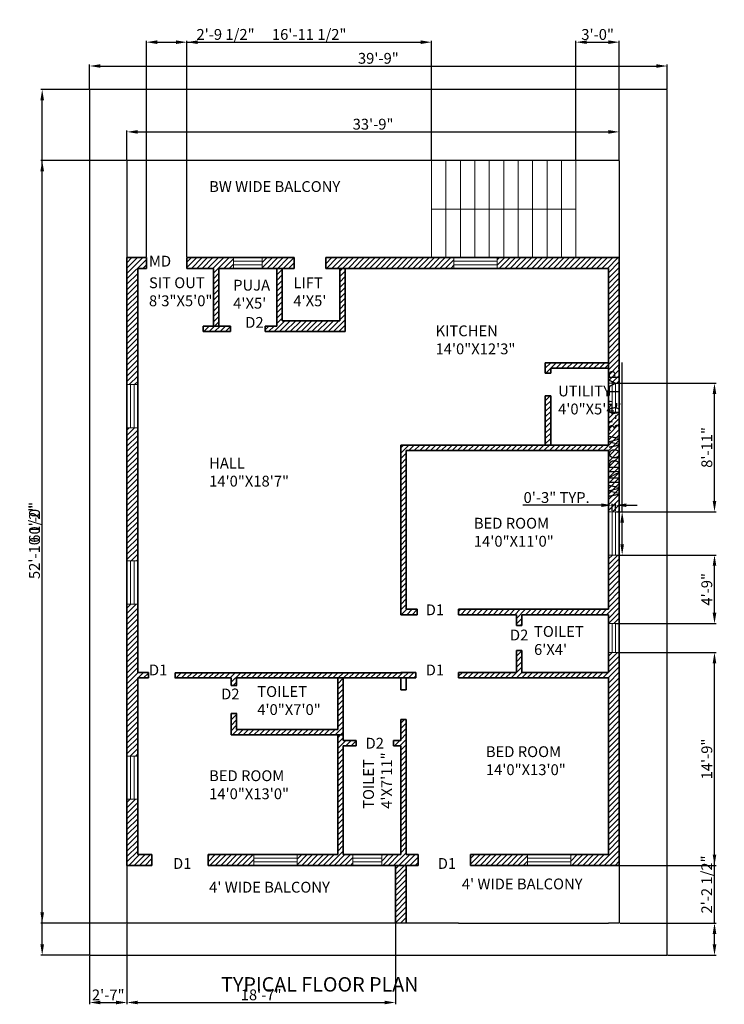
# Model space of a CAD drawing. Units: inches. Extents: x 9573 to 10767, y 4927 to 5746.
# Tile 1 of 2: x 9573 to 10158, y 4927 to 5746. Entities that reach past the tile are written whole.
import ezdxf

# ---------------------------------------------------------------- set-up
doc = ezdxf.new("R2010")
doc.units = ezdxf.units.IN
for name, color, linetype, lineweight in [('A-ANNO-DIMS', 2, 'Continuous', 18), ('A-ANNO-TEXT', 7, 'Continuous', 25), ('A-AREA-IDEN', 7, 'Continuous', 18), ('A-DOOR-IDEN', 3, 'Continuous', 18), ('A-FLOR-BALC', 7, 'Continuous', 25), ('A-FLOR-STRS', 7, 'Continuous', 18), ('A-GLAZ', 4, 'Continuous', 18), ('A-WALL', 7, 'Continuous', 35), ('A-WALL-PATT', 252, 'Continuous', 13), ('C-PROP', 8, 'Continuous', 25)]:
    doc.layers.add(name, color=color, linetype=linetype, lineweight=lineweight)
doc.styles.get("Standard").update_dxf_attribs({"font": 'arial.ttf'})
doc.dimstyles.new('ISO-25', dxfattribs={"dimtxt": 9, "dimasz": 9, "dimexe": 1.25, "dimexo": 0.625, "dimtad": 1, "dimdec": 1, "dimrnd": 9, "dimlunit": 3, "dimtxsty": 'Standard', "dimcen": 2.5, "dimadec": 0, "dimazin": 0, "dimtfac": 1, "dimtdec": 1, "dimtmove": 0, "dimatfit": 3, "dimfxl": 1, "dimarcsym": 0})

# ---------------------------------------------------------------- blocks, each defined once
blk = doc.blocks.new('*D1')
at = {"layer": 'A-ANNO-DIMS', "color": 0, "lineweight": -2, "transparency": 16777216}
for p, q in [((9661.65, 5629.81), (9661.65, 5654.25)), ((9670.65, 5653), (10061.84, 5653)), ((10070.84, 5629.81), (10070.84, 5654.25))]:
    blk.add_line(p, q, dxfattribs=at)
at = {"layer": 'A-ANNO-DIMS', "color": 0, "transparency": 16777216}
for points in [[(9670.65, 5654.5), (9670.65, 5651.5), (9661.65, 5653)], [(10061.84, 5654.5), (10061.84, 5651.5), (10070.84, 5653)]]:
    blk.add_solid(points, dxfattribs=at)
at = {"layer": 'Defpoints', "color": 0, "transparency": 16777216}
for p in [(10070.84, 5653), (9661.65, 5629.18), (10070.84, 5629.18)]:
    blk.add_point(p, dxfattribs=at)
at = {"layer": 'A-ANNO-DIMS', "color": 0, "transparency": 16777216, "insert": (9866.24, 5658.23), "char_height": 9, "attachment_point": 5}
blk.add_mtext('33\'-9"', dxfattribs=at)
blk = doc.blocks.new('*D2')
at = {"layer": 'A-ANNO-DIMS', "color": 0, "lineweight": -2, "transparency": 16777216}
for p, q in [((9630.63, 5688.89), (9630.63, 5709.04)), ((9639.63, 5707.79), (10101.63, 5707.79)), ((10110.63, 5688.89), (10110.63, 5709.04))]:
    blk.add_line(p, q, dxfattribs=at)
at = {"layer": 'A-ANNO-DIMS', "color": 0, "transparency": 16777216}
for points in [[(9639.63, 5709.29), (9639.63, 5706.29), (9630.63, 5707.79)], [(10101.63, 5709.29), (10101.63, 5706.29), (10110.63, 5707.79)]]:
    blk.add_solid(points, dxfattribs=at)
at = {"layer": 'Defpoints', "color": 0, "transparency": 16777216}
for p in [(10110.63, 5707.79), (9630.63, 5688.26), (10110.63, 5688.26)]:
    blk.add_point(p, dxfattribs=at)
at = {"layer": 'A-ANNO-DIMS', "color": 0, "transparency": 16777216, "insert": (9870.63, 5713.01), "char_height": 9, "attachment_point": 5}
blk.add_mtext('39\'-9"', dxfattribs=at)
blk = doc.blocks.new('GLAZ-36IN')
for p, q in [((0, 3), (36, 3)), ((0, 0), (36, 0))]:
    blk.add_line(p, q)
blk = doc.blocks.new('GLAZ-24IN')
for p, q in [((0, 3), (24, 3)), ((0, 0), (24, 0))]:
    blk.add_line(p, q)
blk = doc.blocks.new('STAIR-TWIN-FLIGHT')
for p, q in [((0, 80.77), (0, 0)), ((12, 80.77), (12, 0)), ((24, 80.77), (24, 0)), ((36, 80.77), (36, 0)), ((48, 80.77), (48, 0)), ((60, 80.77), (60, 0)), ((72, 80.77), (72, 0)), ((84, 80.77), (84, 0)), ((96, 80.77), (96, 0)), ((108, 80.77), (108, 0)), ((120, 80.77), (120, 0)), ((0, 40.39), (120, 40.39))]:
    blk.add_line(p, q)
blk = doc.blocks.new('*D8')
at = {"layer": 'A-ANNO-DIMS', "color": 0, "lineweight": -2, "transparency": 16777216}
for p, q in [((10073.24, 5337.09), (10073.24, 5461.23)), ((10068.46, 5337.09), (10074.49, 5337.09)), ((10073.24, 5310.09), (10073.24, 5328.09)), ((10068.46, 5301.09), (10074.49, 5301.09))]:
    blk.add_line(p, q, dxfattribs=at)
at = {"layer": 'A-ANNO-DIMS', "color": 0, "transparency": 16777216}
for points in [[(10071.74, 5328.09), (10074.74, 5328.09), (10073.24, 5337.09)], [(10071.74, 5310.09), (10074.74, 5310.09), (10073.24, 5301.09)]]:
    blk.add_solid(points, dxfattribs=at)
at = {"layer": 'Defpoints', "color": 0, "transparency": 16777216}
for p in [(10067.84, 5337.09), (10073.24, 5337.09), (10067.84, 5301.09)]:
    blk.add_point(p, dxfattribs=at)
at = {"layer": 'A-ANNO-DIMS', "color": 0, "transparency": 16777216, "insert": (10067.95, 5403.66), "char_height": 9, "attachment_point": 5, "rotation": 90}
blk.add_mtext('WINDOW 3\'-0" TYP.', dxfattribs=at)
blk = doc.blocks.new('*D9')
at = {"layer": 'A-ANNO-DIMS', "color": 0, "lineweight": -2, "transparency": 16777216}
for p, q in [((10055.84, 5342.49), (9990.73, 5342.49)), ((10064.84, 5337.72), (10064.84, 5343.74)), ((10067.84, 5342.49), (10064.84, 5342.49)), ((10067.84, 5337.72), (10067.84, 5343.74)), ((10076.84, 5342.49), (10085.84, 5342.49))]:
    blk.add_line(p, q, dxfattribs=at)
at = {"layer": 'A-ANNO-DIMS', "color": 0, "transparency": 16777216}
for points in [[(10055.84, 5343.99), (10055.84, 5340.99), (10064.84, 5342.49)], [(10076.84, 5343.99), (10076.84, 5340.99), (10067.84, 5342.49)]]:
    blk.add_solid(points, dxfattribs=at)
at = {"layer": 'Defpoints', "color": 0, "transparency": 16777216}
for p in [(10064.84, 5342.49), (10064.84, 5337.09), (10067.84, 5337.09)]:
    blk.add_point(p, dxfattribs=at)
at = {"layer": 'A-ANNO-DIMS', "color": 0, "transparency": 16777216, "insert": (10018.78, 5347.72), "char_height": 9, "attachment_point": 5}
blk.add_mtext('0\'-3" TYP.', dxfattribs=at)
blk = doc.blocks.new('*D14')
at = {"layer": 'A-ANNO-DIMS', "color": 0, "lineweight": -2, "transparency": 16777216}
for p, q in [((9661.02, 5629.18), (9590.03, 5629.18)), ((9591.28, 5003.91), (9591.28, 5620.18)), ((9661.02, 4994.91), (9590.03, 4994.91))]:
    blk.add_line(p, q, dxfattribs=at)
at = {"layer": 'A-ANNO-DIMS', "color": 0, "transparency": 16777216}
for points in [[(9589.78, 5620.18), (9592.78, 5620.18), (9591.28, 5629.18)], [(9589.78, 5003.91), (9592.78, 5003.91), (9591.28, 4994.91)]]:
    blk.add_solid(points, dxfattribs=at)
at = {"layer": 'Defpoints', "color": 0, "transparency": 16777216}
for p in [(9591.28, 5629.18), (9661.65, 5629.18), (9661.65, 4994.91)]:
    blk.add_point(p, dxfattribs=at)
at = {"layer": 'A-ANNO-DIMS', "color": 0, "transparency": 16777216, "insert": (9586, 5312.05), "char_height": 9, "attachment_point": 5, "rotation": 90}
blk.add_mtext('52\'-10 1/2"', dxfattribs=at)
blk = doc.blocks.new('*D15')
at = {"layer": 'A-ANNO-DIMS', "color": 0, "lineweight": -2, "transparency": 16777216}
for p, q in [((9630, 5688.26), (9590.03, 5688.26)), ((9591.28, 4977.26), (9591.28, 5679.26)), ((9630, 4968.26), (9590.03, 4968.26))]:
    blk.add_line(p, q, dxfattribs=at)
at = {"layer": 'A-ANNO-DIMS', "color": 0, "transparency": 16777216}
for points in [[(9589.78, 5679.26), (9592.78, 5679.26), (9591.28, 5688.26)], [(9589.78, 4977.26), (9592.78, 4977.26), (9591.28, 4968.26)]]:
    blk.add_solid(points, dxfattribs=at)
at = {"layer": 'Defpoints', "color": 0, "transparency": 16777216}
for p in [(9591.28, 5688.26), (9630.63, 5688.26), (9630.63, 4968.26)]:
    blk.add_point(p, dxfattribs=at)
at = {"layer": 'A-ANNO-DIMS', "color": 0, "transparency": 16777216, "insert": (9586.06, 5328.26), "char_height": 9, "attachment_point": 5, "rotation": 90}
blk.add_mtext('60\'-0"', dxfattribs=at)
blk = doc.blocks.new('*D16')
at = {"layer": 'A-ANNO-DIMS', "color": 0, "lineweight": -2, "transparency": 16777216}
for p, q in [((9661.65, 4994.28), (9661.65, 4927.66)), ((9630.63, 4967.64), (9630.63, 4927.66)), ((9639.63, 4928.91), (9652.65, 4928.91))]:
    blk.add_line(p, q, dxfattribs=at)
at = {"layer": 'A-ANNO-DIMS', "color": 0, "transparency": 16777216}
for points in [[(9639.63, 4930.41), (9639.63, 4927.41), (9630.63, 4928.91)], [(9652.65, 4930.41), (9652.65, 4927.41), (9661.65, 4928.91)]]:
    blk.add_solid(points, dxfattribs=at)
at = {"layer": 'Defpoints', "color": 0, "transparency": 16777216}
for p in [(9661.65, 4994.91), (9630.63, 4968.26), (9661.65, 4928.91)]:
    blk.add_point(p, dxfattribs=at)
at = {"layer": 'A-ANNO-DIMS', "color": 0, "transparency": 16777216, "insert": (9646.14, 4934.06), "char_height": 9, "attachment_point": 5}
blk.add_mtext('2\'-7"', dxfattribs=at)
blk = doc.blocks.new('*D17')
at = {"layer": 'A-ANNO-DIMS', "color": 0, "lineweight": -2, "transparency": 16777216}
for p, q in [((10149.98, 4994.91), (10149.98, 5050.21)), ((10071.46, 4994.91), (10151.23, 4994.91)), ((10149.98, 4977.26), (10149.98, 4985.91)), ((10111.25, 4968.26), (10151.23, 4968.26))]:
    blk.add_line(p, q, dxfattribs=at)
at = {"layer": 'A-ANNO-DIMS', "color": 0, "transparency": 16777216}
for points in [[(10148.48, 4985.91), (10151.48, 4985.91), (10149.98, 4994.91)], [(10148.48, 4977.26), (10151.48, 4977.26), (10149.98, 4968.26)]]:
    blk.add_solid(points, dxfattribs=at)
at = {"layer": 'Defpoints', "color": 0, "transparency": 16777216}
for p in [(10070.84, 4994.91), (10149.98, 4994.91), (10110.63, 4968.26)]:
    blk.add_point(p, dxfattribs=at)
at = {"layer": 'A-ANNO-DIMS', "color": 0, "transparency": 16777216, "insert": (10144.7, 5027.06), "char_height": 9, "attachment_point": 5, "rotation": 90}
blk.add_mtext('2\'-2 1/2"', dxfattribs=at)
blk = doc.blocks.new('*D22')
at = {"layer": 'A-ANNO-DIMS', "color": 0, "lineweight": -2, "transparency": 16777216}
for p, q in [((10034.84, 5629.81), (10034.84, 5728.86)), ((10043.84, 5727.61), (10061.84, 5727.61)), ((10070.84, 5629.81), (10070.84, 5728.86))]:
    blk.add_line(p, q, dxfattribs=at)
at = {"layer": 'A-ANNO-DIMS', "color": 0, "transparency": 16777216}
for points in [[(10043.84, 5729.11), (10043.84, 5726.11), (10034.84, 5727.61)], [(10061.84, 5729.11), (10061.84, 5726.11), (10070.84, 5727.61)]]:
    blk.add_solid(points, dxfattribs=at)
at = {"layer": 'Defpoints', "color": 0, "transparency": 16777216}
for p in [(10070.84, 5727.61), (10034.84, 5629.18), (10070.84, 5629.18)]:
    blk.add_point(p, dxfattribs=at)
at = {"layer": 'A-ANNO-DIMS', "color": 0, "transparency": 16777216, "insert": (10052.84, 5732.83), "char_height": 9, "attachment_point": 5}
blk.add_mtext('3\'-0"', dxfattribs=at)
blk = doc.blocks.new('*D24')
at = {"layer": 'A-ANNO-DIMS', "color": 0, "lineweight": -2, "transparency": 16777216}
for p, q in [((9677.83, 5549.03), (9677.83, 5728.86)), ((9686.83, 5727.61), (9702.46, 5727.61)), ((9711.46, 5549.03), (9711.46, 5728.86)), ((9711.46, 5727.61), (9766.76, 5727.61))]:
    blk.add_line(p, q, dxfattribs=at)
at = {"layer": 'A-ANNO-DIMS', "color": 0, "transparency": 16777216}
for points in [[(9686.83, 5729.11), (9686.83, 5726.11), (9677.83, 5727.61)], [(9702.46, 5729.11), (9702.46, 5726.11), (9711.46, 5727.61)]]:
    blk.add_solid(points, dxfattribs=at)
at = {"layer": 'Defpoints', "color": 0, "transparency": 16777216}
for p in [(9711.46, 5727.61), (9677.83, 5548.41), (9711.46, 5548.41)]:
    blk.add_point(p, dxfattribs=at)
at = {"layer": 'A-ANNO-DIMS', "color": 0, "transparency": 16777216, "insert": (9743.61, 5732.89), "char_height": 9, "attachment_point": 5}
blk.add_mtext('2\'-9 1/2"', dxfattribs=at)
blk = doc.blocks.new('*D25')
at = {"layer": 'A-ANNO-DIMS', "color": 0, "lineweight": -2, "transparency": 16777216}
for p, q in [((9711.46, 5549.03), (9711.46, 5728.86)), ((9720.46, 5727.61), (9905.84, 5727.61)), ((9914.84, 5629.81), (9914.84, 5728.86))]:
    blk.add_line(p, q, dxfattribs=at)
at = {"layer": 'A-ANNO-DIMS', "color": 0, "transparency": 16777216}
for points in [[(9720.46, 5729.11), (9720.46, 5726.11), (9711.46, 5727.61)], [(9905.84, 5729.11), (9905.84, 5726.11), (9914.84, 5727.61)]]:
    blk.add_solid(points, dxfattribs=at)
at = {"layer": 'Defpoints', "color": 0, "transparency": 16777216}
for p in [(9914.84, 5727.61), (9914.84, 5629.18), (9711.46, 5548.41)]:
    blk.add_point(p, dxfattribs=at)
at = {"layer": 'A-ANNO-DIMS', "color": 0, "transparency": 16777216, "insert": (9813.15, 5732.89), "char_height": 9, "attachment_point": 5}
blk.add_mtext('16\'-11 1/2"', dxfattribs=at)
blk = doc.blocks.new('*D28')
at = {"layer": 'A-ANNO-DIMS', "color": 0, "lineweight": -2, "transparency": 16777216}
for p, q in [((10068.46, 5220), (10151.23, 5220)), ((10149.98, 5051.91), (10149.98, 5211)), ((10071.46, 5042.91), (10151.23, 5042.91))]:
    blk.add_line(p, q, dxfattribs=at)
at = {"layer": 'A-ANNO-DIMS', "color": 0, "transparency": 16777216}
for points in [[(10148.48, 5211), (10151.48, 5211), (10149.98, 5220)], [(10148.48, 5051.91), (10151.48, 5051.91), (10149.98, 5042.91)]]:
    blk.add_solid(points, dxfattribs=at)
at = {"layer": 'Defpoints', "color": 0, "transparency": 16777216}
for p in [(10067.84, 5220), (10149.98, 5220), (10070.84, 5042.91)]:
    blk.add_point(p, dxfattribs=at)
at = {"layer": 'A-ANNO-DIMS', "color": 0, "transparency": 16777216, "insert": (10144.76, 5131.45), "char_height": 9, "attachment_point": 5, "rotation": 90}
blk.add_mtext('14\'-9"', dxfattribs=at)
blk = doc.blocks.new('*D29')
at = {"layer": 'A-ANNO-DIMS', "color": 0, "lineweight": -2, "transparency": 16777216}
for p, q in [((10068.46, 5301.09), (10151.23, 5301.09)), ((10149.98, 5253), (10149.98, 5292.09)), ((10068.46, 5244), (10151.23, 5244))]:
    blk.add_line(p, q, dxfattribs=at)
at = {"layer": 'A-ANNO-DIMS', "color": 0, "transparency": 16777216}
for points in [[(10148.48, 5292.09), (10151.48, 5292.09), (10149.98, 5301.09)], [(10148.48, 5253), (10151.48, 5253), (10149.98, 5244)]]:
    blk.add_solid(points, dxfattribs=at)
at = {"layer": 'Defpoints', "color": 0, "transparency": 16777216}
for p in [(10067.84, 5301.09), (10149.98, 5301.09), (10067.84, 5244)]:
    blk.add_point(p, dxfattribs=at)
at = {"layer": 'A-ANNO-DIMS', "color": 0, "transparency": 16777216, "insert": (10144.76, 5272.55), "char_height": 9, "attachment_point": 5, "rotation": 90}
blk.add_mtext('4\'-9"', dxfattribs=at)
blk = doc.blocks.new('*D30')
at = {"layer": 'A-ANNO-DIMS', "color": 0, "lineweight": -2, "transparency": 16777216}
for p, q in [((10068.46, 5444), (10151.23, 5444)), ((10149.98, 5346.09), (10149.98, 5435)), ((10068.46, 5337.09), (10151.23, 5337.09))]:
    blk.add_line(p, q, dxfattribs=at)
at = {"layer": 'A-ANNO-DIMS', "color": 0, "transparency": 16777216}
for points in [[(10148.48, 5435), (10151.48, 5435), (10149.98, 5444)], [(10148.48, 5346.09), (10151.48, 5346.09), (10149.98, 5337.09)]]:
    blk.add_solid(points, dxfattribs=at)
at = {"layer": 'Defpoints', "color": 0, "transparency": 16777216}
for p in [(10067.84, 5444), (10149.98, 5444), (10067.84, 5337.09)]:
    blk.add_point(p, dxfattribs=at)
at = {"layer": 'A-ANNO-DIMS', "color": 0, "transparency": 16777216, "insert": (10144.76, 5390.55), "char_height": 9, "attachment_point": 5, "rotation": 90}
blk.add_mtext('8\'-11"', dxfattribs=at)
blk = doc.blocks.new('*D34')
at = {"layer": 'A-ANNO-DIMS', "color": 0, "lineweight": -2, "transparency": 16777216}
for p, q in [((9661.65, 4994.28), (9661.65, 4927.66)), ((9884.84, 4994.28), (9884.84, 4927.66)), ((9670.65, 4928.91), (9875.84, 4928.91))]:
    blk.add_line(p, q, dxfattribs=at)
at = {"layer": 'A-ANNO-DIMS', "color": 0, "transparency": 16777216}
for points in [[(9670.65, 4930.41), (9670.65, 4927.41), (9661.65, 4928.91)], [(9875.84, 4930.41), (9875.84, 4927.41), (9884.84, 4928.91)]]:
    blk.add_solid(points, dxfattribs=at)
at = {"layer": 'Defpoints', "color": 0, "transparency": 16777216}
for p in [(9661.65, 4994.91), (9884.84, 4994.91), (9884.84, 4928.91)]:
    blk.add_point(p, dxfattribs=at)
at = {"layer": 'A-ANNO-DIMS', "color": 0, "transparency": 16777216, "insert": (9773.24, 4934.13), "char_height": 9, "attachment_point": 5}
blk.add_mtext('18\'-7"', dxfattribs=at)

msp = doc.modelspace()

# ---------------------------------------------------------------- hatches: boundary and pattern name
at = {"layer": 'A-WALL-PATT'}
h = msp.add_hatch(dxfattribs=at)
h.set_pattern_fill('ANSI31', color=256)
h.paths.add_polyline_path([(9800.61, 5548.41), (9774.15, 5548.41), (9774.15, 5539.41), (9800.61, 5539.41)])
h.paths.add_polyline_path([(9790.65, 5539.41), (9786.15, 5539.41), (9786.15, 5491.41), (9776.56, 5491.41), (9776.56, 5486.91), (9790.65, 5486.91), (9843.15, 5486.91), (9843.15, 5539.41), (9838.65, 5539.41), (9838.65, 5495.91), (9790.65, 5495.91)])
h.paths.add_polyline_path([(9747.85, 5491.41), (9725.13, 5491.41), (9725.13, 5486.91), (9747.85, 5486.91)])
h.paths.add_polyline_path([(9933.39, 5548.41), (9826.9, 5548.41), (9826.9, 5539.41), (9933.39, 5539.41)])
h.paths.add_polyline_path([(10070.84, 5548.41), (9969.39, 5548.41), (9969.39, 5539.41), (10061.84, 5539.41), (10061.84, 5444), (10070.84, 5444)])
h.paths.add_polyline_path([(10070.84, 5420), (10061.84, 5420), (10061.84, 5392.41), (9889.34, 5392.41), (9889.34, 5251.41), (9902.98, 5251.41), (9902.98, 5255.91), (9893.84, 5255.91), (9893.84, 5387.91), (10061.84, 5387.91), (10061.84, 5337.09), (10070.84, 5337.09)])
h.paths.add_polyline_path([(10013.84, 5433.61), (10009.34, 5433.61), (10009.34, 5392.41), (10013.84, 5392.41)])
h.paths.add_polyline_path([(10061.84, 5460.91), (10009.34, 5460.91), (10009.34, 5452.41), (10013.84, 5452.41), (10013.84, 5456.41), (10061.84, 5456.41)], flags=17)
h.paths.add_polyline_path([(9670.65, 5406.85), (9661.65, 5406.85), (9661.65, 5296.18), (9670.65, 5296.18)])
h.paths.add_polyline_path([(9670.65, 5486.91), (9670.65, 5491.41), (9670.65, 5539.41), (9677.83, 5539.41), (9677.83, 5548.41), (9661.65, 5548.41), (9661.65, 5442.85), (9670.65, 5442.85)])
h.paths.add_polyline_path([(9682.45, 5051.91), (9670.65, 5051.91), (9670.65, 5097.91), (9661.65, 5097.91), (9661.65, 5065.4), (9661.65, 5042.91), (9682.45, 5042.91)])
h.paths.add_polyline_path([(9841.34, 5198.91), (9836.84, 5198.91), (9836.84, 5155.91), (9752.84, 5155.91), (9752.84, 5169.21), (9748.34, 5169.21), (9748.34, 5151.41), (9841.34, 5151.41)])
h = msp.add_hatch(dxfattribs=at)
h.set_pattern_fill('ANSI31', color=256)
h.paths.add_polyline_path([(9767.07, 5051.91), (9729.1, 5051.91), (9729.1, 5042.91), (9767.07, 5042.91)])
h.paths.add_polyline_path([(9670.65, 5198.91), (9679.58, 5198.91), (9679.58, 5203.27), (9670.65, 5203.26), (9670.65, 5260.18), (9661.65, 5260.18), (9661.65, 5133.91), (9670.65, 5133.91)])
h.paths.add_polyline_path([(9849.48, 5051.91), (9841.34, 5051.91), (9841.34, 5142.41), (9852.17, 5142.41), (9852.17, 5146.91), (9841.34, 5146.91), (9841.34, 5151.41), (9836.84, 5151.41), (9836.84, 5051.91), (9803.07, 5051.91), (9803.07, 5042.91), (9849.48, 5042.91)])
h.paths.add_polyline_path([(9901.78, 5203.41), (9889.34, 5203.4), (9889.34, 5203.23), (9701.87, 5203.23), (9701.87, 5198.91), (9748.34, 5198.91), (9748.34, 5192.53), (9752.84, 5192.53), (9752.84, 5198.91), (9901.78, 5198.91)])
h.paths.add_polyline_path([(9893.84, 5164.29), (9889.34, 5164.29), (9889.34, 5146.91), (9883.18, 5146.91), (9883.18, 5142.41), (9889.34, 5142.41), (9889.34, 5051.91), (9873.48, 5051.91), (9873.48, 5042.91), (9903.59, 5042.91), (9903.59, 5051.91), (9893.84, 5051.91)])
h.paths.add_polyline_path([(9893.84, 5042.91), (9884.84, 5042.91), (9884.84, 4994.91), (9893.84, 4994.91)])
h.paths.add_polyline_path([(9994.59, 5051.91), (9947.29, 5051.91), (9947.29, 5042.91), (9994.59, 5042.91)], flags=17)
h.paths.add_polyline_path([(10070.84, 5065.4), (10070.84, 5220), (10061.84, 5220), (10061.84, 5203.41), (9989.84, 5203.41), (9989.84, 5221.8), (9985.34, 5221.8), (9985.34, 5203.41), (9937.34, 5203.41), (9937.34, 5198.91), (10061.84, 5198.91), (10061.84, 5051.91), (10030.59, 5051.91), (10030.59, 5042.91), (10061.84, 5042.91), (10070.84, 5042.91)])
h.paths.add_polyline_path([(10070.84, 5301.09), (10061.84, 5301.09), (10061.84, 5255.91), (9937.34, 5255.91), (9937.34, 5251.41), (9985.34, 5251.41), (9985.34, 5242.53), (9989.84, 5242.53), (9989.84, 5251.41), (10061.84, 5251.41), (10061.84, 5244), (10070.84, 5244)])
h.paths.add_polyline_path([(9750.15, 5548.41), (9711.46, 5548.41), (9711.46, 5539.41), (9733.65, 5539.41), (9733.65, 5491.41), (9738.15, 5491.41), (9738.15, 5539.41), (9750.15, 5539.41)])

# ---------------------------------------------------------------- linework, layer by layer
at = {"layer": 'A-FLOR-BALC'}
for p, q in [((10070.84, 5629.18), (9661.65, 5629.18)), ((9661.65, 5629.18), (9661.65, 5548.41)), ((10070.84, 5629.18), (10070.84, 5548.41)), ((9661.65, 5042.91), (9661.65, 4994.91)), ((10070.84, 5042.91), (10070.84, 4994.91)), ((9937.34, 4994.91), (9661.65, 4994.91)), ((9937.34, 4994.91), (10061.84, 4994.91)), ((10070.84, 4994.91), (10061.84, 4994.91))]:
    msp.add_line(p, q, dxfattribs=at)
at = {"layer": 'A-GLAZ'}
for p, q in [((9750.15, 5548.41), (9750.15, 5539.41)), ((9774.15, 5548.41), (9774.15, 5539.41)), ((9933.39, 5548.41), (9933.39, 5539.41)), ((9969.39, 5548.41), (9969.39, 5539.41)), ((9670.65, 5442.85), (9661.65, 5442.85)), ((10061.84, 5444), (10070.84, 5444)), ((10061.84, 5420), (10070.84, 5420)), ((9670.65, 5406.85), (9661.65, 5406.85)), ((10070.84, 5337.09), (10061.84, 5337.09)), ((10070.84, 5301.09), (10061.84, 5301.09)), ((9670.65, 5296.18), (9661.65, 5296.18)), ((9670.65, 5260.18), (9661.65, 5260.18)), ((10061.84, 5244), (10070.84, 5244)), ((10061.84, 5220), (10070.84, 5220)), ((9670.65, 5133.91), (9661.65, 5133.91)), ((9670.65, 5097.91), (9661.65, 5097.91)), ((9767.07, 5051.91), (9767.07, 5042.91)), ((9803.07, 5051.91), (9803.07, 5042.91)), ((9849.48, 5051.91), (9849.48, 5042.91)), ((9873.48, 5051.91), (9873.48, 5042.91)), ((9994.59, 5051.91), (9994.59, 5042.91)), ((10030.59, 5051.91), (10030.59, 5042.91))]:
    msp.add_line(p, q, dxfattribs=at)
at = {"layer": 'A-WALL'}
for p, q in [((9661.65, 5548.41), (9677.83, 5548.41)), ((9661.65, 5548.41), (9661.65, 5065.4)), ((9677.83, 5548.41), (9677.83, 5539.41)), ((9711.46, 5548.41), (9711.46, 5539.41)), ((9711.46, 5548.41), (9800.61, 5548.41)), ((9800.61, 5548.41), (9800.61, 5539.41)), ((9826.9, 5548.41), (9826.9, 5539.41)), ((9826.9, 5548.41), (10070.84, 5548.41)), ((9670.65, 5539.41), (9677.83, 5539.41)), ((9711.46, 5539.41), (9733.65, 5539.41)), ((9738.15, 5539.41), (9800.61, 5539.41)), ((9826.9, 5539.41), (10061.84, 5539.41)), ((9838.65, 5495.91), (9790.65, 5495.91)), ((9670.65, 5491.41), (9670.65, 5486.91)), ((9670.65, 5486.91), (9670.65, 5203.26)), ((9725.13, 5491.41), (9747.85, 5491.41)), ((9725.13, 5491.41), (9725.13, 5486.91)), ((9725.13, 5486.91), (9747.85, 5486.91)), ((9747.85, 5491.41), (9747.85, 5486.91)), ((9776.56, 5491.41), (9776.56, 5486.91)), ((9776.56, 5491.41), (9786.15, 5491.41)), ((9776.56, 5486.91), (9790.65, 5486.91)), ((9843.15, 5486.91), (9790.65, 5486.91)), ((10009.34, 5460.91), (10061.84, 5460.91)), ((10013.84, 5456.41), (10061.84, 5456.41)), ((10013.84, 5452.41), (10009.34, 5452.41)), ((10013.84, 5433.61), (10009.34, 5433.61)), ((9889.34, 5392.41), (10061.84, 5392.41)), ((9893.84, 5387.91), (10061.84, 5387.91)), ((9889.34, 5251.41), (9902.98, 5251.41)), ((9893.84, 5255.91), (9902.98, 5255.91)), ((9902.98, 5255.91), (9902.98, 5251.41)), ((9937.34, 5255.91), (9937.34, 5251.41)), ((9937.34, 5255.91), (10061.84, 5255.91)), ((9937.34, 5251.41), (9985.34, 5251.41)), ((9989.84, 5251.41), (10061.84, 5251.41)), ((9985.34, 5242.53), (9989.84, 5242.53)), ((9985.34, 5221.8), (9989.84, 5221.8)), ((9679.58, 5203.27), (9670.57, 5203.26)), ((9670.65, 5203.26), (9670.57, 5203.26)), ((9679.58, 5203.27), (9679.58, 5198.9)), ((9701.87, 5203.23), (9701.87, 5198.78)), ((9701.87, 5203.23), (9889.34, 5203.23)), ((9889.34, 5203.41), (9889.34, 5203.23)), ((9901.78, 5203.41), (9889.34, 5203.4)), ((9901.78, 5203.41), (9901.78, 5198.91)), ((9937.34, 5203.41), (9985.34, 5203.41)), ((9937.34, 5203.41), (9937.34, 5198.91)), ((9989.84, 5203.41), (10061.84, 5203.41)), ((9679.58, 5198.91), (9670.65, 5198.91)), ((9670.65, 5198.91), (9670.65, 5051.91)), ((9748.34, 5198.91), (9701.87, 5198.91)), ((9748.19, 5192.53), (9753.04, 5192.53)), ((9748.34, 5192.53), (9748.34, 5198.91)), ((9901.78, 5198.91), (9752.84, 5198.91)), ((9752.84, 5192.53), (9752.84, 5198.91)), ((9836.84, 5155.91), (9836.84, 5198.91)), ((9841.34, 5146.91), (9841.34, 5198.91)), ((9889.34, 5189.03), (9889.34, 5198.91)), ((9893.84, 5189.03), (9893.84, 5198.91)), ((9937.34, 5198.91), (10061.84, 5198.91)), ((10061.84, 5051.91), (10061.84, 5198.91)), ((9889.34, 5189.03), (9893.84, 5189.03)), ((9748.19, 5169.21), (9753.04, 5169.21)), ((9748.34, 5151.41), (9748.34, 5169.21)), ((9752.84, 5155.91), (9752.84, 5169.21)), ((9889.34, 5164.29), (9893.84, 5164.29)), ((9889.34, 5146.91), (9889.34, 5164.29)), ((9893.84, 5051.91), (9893.84, 5164.29)), ((9841.34, 5151.41), (9748.34, 5151.41)), ((9836.84, 5155.91), (9752.84, 5155.91)), ((9836.84, 5051.91), (9836.84, 5151.41)), ((9852.17, 5146.91), (9841.34, 5146.91)), ((9852.17, 5146.91), (9852.17, 5142.41)), ((9889.34, 5146.91), (9883.18, 5146.91)), ((9883.18, 5146.91), (9883.18, 5142.41)), ((9841.34, 5051.91), (9841.34, 5142.41)), ((9852.17, 5142.41), (9841.34, 5142.41)), ((9889.34, 5142.41), (9883.18, 5142.41)), ((9889.34, 5051.91), (9889.34, 5142.41)), ((9661.65, 5042.91), (9661.65, 5065.4)), ((10070.84, 5065.4), (10070.84, 5042.91)), ((9682.45, 5051.91), (9670.65, 5051.91)), ((9682.45, 5051.91), (9682.45, 5042.91)), ((9836.84, 5051.91), (9729.1, 5051.91)), ((9729.1, 5051.91), (9729.1, 5042.91)), ((9889.34, 5051.91), (9841.34, 5051.91)), ((9903.59, 5051.91), (9893.84, 5051.91)), ((9903.59, 5051.91), (9903.59, 5042.91)), ((9947.29, 5051.91), (10061.84, 5051.91)), ((9947.29, 5051.91), (9947.29, 5042.91)), ((9682.45, 5042.91), (9661.65, 5042.91)), ((9903.59, 5042.91), (9729.1, 5042.91)), ((9884.84, 4994.91), (9884.84, 5042.91)), ((9893.84, 4994.91), (9893.84, 5042.91)), ((9947.29, 5042.91), (10061.84, 5042.91)), ((10070.84, 5042.91), (10061.84, 5042.91))]:
    msp.add_line(p, q, dxfattribs=at)
for points in [[(10070.84, 5548.41), (10070.84, 5065.4)], [(9670.65, 5491.41), (9670.65, 5539.41)], [(9733.65, 5491.41), (9733.65, 5539.41)], [(9738.15, 5491.41), (9738.15, 5539.41)], [(9786.15, 5491.41), (9786.15, 5539.41)], [(9790.65, 5495.91), (9790.65, 5539.41)], [(9838.65, 5495.91), (9838.65, 5539.41)], [(9843.15, 5486.91), (9843.15, 5539.41)], [(10061.84, 5539.41), (10061.84, 5392.41)], [(10009.34, 5460.91), (10009.34, 5452.41)], [(10013.84, 5456.41), (10013.84, 5452.41)], [(10009.34, 5433.61), (10009.34, 5392.41)], [(10013.84, 5433.61), (10013.84, 5392.41)], [(9889.34, 5392.41), (9889.34, 5251.41)], [(9893.84, 5387.91), (9893.84, 5255.91)], [(10061.84, 5387.91), (10061.84, 5255.91)], [(9985.34, 5251.41), (9985.34, 5242.53)], [(9989.84, 5251.41), (9989.84, 5242.53)], [(10061.84, 5251.41), (10061.84, 5203.41)], [(9985.34, 5221.8), (9985.34, 5203.41)], [(9989.84, 5221.8), (9989.84, 5203.41)]]:
    msp.add_lwpolyline(points, dxfattribs=at)
at = {"layer": 'C-PROP'}
for p, q in [((10110.63, 5688.26), (9630.63, 5688.26)), ((9630.63, 5688.26), (9630.63, 4968.26)), ((10110.63, 4968.26), (10110.63, 5688.26)), ((9630.63, 4968.26), (10110.63, 4968.26))]:
    msp.add_line(p, q, dxfattribs=at)

# ---------------------------------------------------------------- block references
at = {"layer": 'A-FLOR-STRS'}
msp.add_blockref('STAIR-TWIN-FLIGHT', (9914.84, 5548.41), dxfattribs=at)
at = {"layer": 'A-GLAZ'}
for name, p in [('GLAZ-24IN', (9750.15, 5542.41)), ('GLAZ-36IN', (9933.39, 5542.41))]:
    msp.add_blockref(name, p, dxfattribs=at)
for name, p, rotation in [('GLAZ-36IN', (9667.64, 5406.85), 90.00000000000286), ('GLAZ-24IN', (10064.84, 5444), 270.0000000000043), ('GLAZ-36IN', (10067.84, 5301.09), 90.00000000000286), ('GLAZ-36IN', (9667.64, 5260.18), 90.0000000000031), ('GLAZ-24IN', (10064.84, 5244), 270.0000000000043), ('GLAZ-36IN', (9667.64, 5097.91), 90.00000000000266), ('GLAZ-36IN', (9803.07, 5048.91), 180), ('GLAZ-24IN', (9873.48, 5048.91), 180), ('GLAZ-36IN', (10030.59, 5048.91), 180)]:
    msp.add_blockref(name, p, dxfattribs=dict(at, rotation=rotation))

# ---------------------------------------------------------------- texts
at = {"layer": 'A-ANNO-TEXT', "insert": (9740, 4950), "char_height": 12, "attachment_point": 1}
msp.add_mtext_dynamic_manual_height_columns('TYPICAL FLOOR PLAN', width=390, gutter_width=12.5, heights=[0], dxfattribs=at)
at = {"layer": 'A-AREA-IDEN', "char_height": 2.5, "attachment_point": 1}
for s, insert in [('{\\H3.6x;BW WIDE BALCONY}', (9730, 5612.02)), ('{\\H3.6x;SIT OUT\\P8\'3"X5\'0"}', (9680, 5532.02)), ("{\\H3.6x;PUJA\\P4'X5'}", (9750, 5530)), ("{\\H3.6x;LIFT\\P4'X5'}", (9800, 5531.99)), ('{\\H3.6x;KITCHEN\\P14\'0"X12\'3"}', (9918.15, 5492.02)), ('{\\H3.6x;UTILITY\\P4\'0"X5\'4"}', (10020, 5442.02)), ('{\\H3.6x;HALL}\\P{\\H3.6x;14\'0"X18\'7"}', (9730, 5382.02)), ('{\\H3.6x;BED ROOM\\P14\'0"X11\'0"}', (9950, 5332.02)), ("{\\H3.6x;TOILET\\P6'X4'}", (10000, 5242.02)), ('{\\H3.6x;TOILET\\P4\'0"X7\'0"}', (9770, 5192.02)), ('{\\H3.6x;BED ROOM\\P14\'0"X13\'0"}', (9960, 5142.02)), ('{\\H3.6x;BED ROOM\\P14\'0"X13\'0"}', (9730, 5122.02)), ("{\\H3.6x;4' WIDE BALCONY}", (9730, 5029.31)), ("{\\H3.6x;4' WIDE BALCONY}", (9940, 5032.02))]:
    msp.add_mtext_dynamic_manual_height_columns(s, width=120, gutter_width=12.5, heights=[0], dxfattribs=dict(at, insert=insert))
at = {"layer": 'A-AREA-IDEN', "insert": (9857.97, 5090), "char_height": 2.5, "attachment_point": 1, "rotation": 90}
msp.add_mtext_dynamic_manual_height_columns('{\\H3.6x;TOILET\\P4\'X7\'11"}', width=120, gutter_width=12.5, heights=[0], dxfattribs=at)
at = {"layer": 'A-DOOR-IDEN', "char_height": 9, "attachment_point": 1}
for s, insert in [('MD', (9680, 5550)), ('D2', (9760, 5499.04)), ('D1', (9910, 5260)), ('D2', (9980, 5239.04)), ('D1', (9680, 5210)), ('D1', (9910, 5210)), ('D2', (9740, 5190)), ('D2', (9860, 5149.04)), ('D1', (9700, 5049.04)), ('D1', (9920, 5049.04))]:
    msp.add_mtext_dynamic_manual_height_columns(s, width=20, gutter_width=12.5, heights=[0], dxfattribs=dict(at, insert=insert))

# ---------------------------------------------------------------- dimensions: what is measured, and where the dimension line sits
at = {"layer": 'A-ANNO-DIMS'}
for base, p1, p2, override, picture, middle in [((9711.46, 5727.61), (9677.83, 5548.41), (9711.46, 5548.41), {"dimdec": 1, "dimlfac": 1, "dimrnd": 0, "dimzin": 1, "dimdsep": 46, "dimlunit": 4, "dimfrac": 2}, '*D24', (9743.61, 5732.89)), ((9914.84, 5727.61), (9711.46, 5548.41), (9914.84, 5629.18), {"dimdec": 1, "dimlfac": 1, "dimrnd": 0, "dimzin": 1, "dimdsep": 46, "dimlunit": 4, "dimfrac": 2}, '*D25', (9813.15, 5732.89)), ((10070.84, 5727.61), (10034.84, 5629.18), (10070.84, 5629.18), {"dimdec": 1, "dimlfac": 1, "dimrnd": 0, "dimzin": 1, "dimdsep": 46, "dimlunit": 4, "dimfrac": 2}, '*D22', (10052.84, 5732.83)), ((10110.63, 5707.79), (9630.63, 5688.26), (10110.63, 5688.26), {"dimclrd": 0, "dimclre": 0, "dimclrt": 0}, '*D2', (9870.63, 5713.01)), ((10070.84, 5653), (9661.65, 5629.18), (10070.84, 5629.18), {"dimclrd": 0, "dimclre": 0, "dimclrt": 0}, '*D1', (9866.24, 5658.23)), ((9661.65, 4928.91), (9630.63, 4968.26), (9661.65, 4994.91), {"dimdec": 1, "dimlfac": 1, "dimrnd": 0, "dimzin": 1, "dimdsep": 46, "dimlunit": 4, "dimfrac": 2}, '*D16', (9646.14, 4934.06)), ((9884.84, 4928.91), (9661.65, 4994.91), (9884.84, 4994.91), {"dimdec": 1, "dimlfac": 1, "dimrnd": 0, "dimzin": 1, "dimdsep": 46, "dimlunit": 4, "dimfrac": 2}, '*D34', (9773.24, 4934.13))]:
    dim = msp.add_linear_dim(base=base, p1=p1, p2=p2, dimstyle='ISO-25', override=override, dxfattribs=at)
    dim.commit()
    dim.dimension.update_dxf_attribs({"geometry": picture, "text_midpoint": middle})
for base, p1, p2, picture, middle in [((9591.28, 5688.26), (9630.63, 4968.26), (9630.63, 5688.26), '*D15', (9586.06, 5328.26)), ((9591.28, 5629.18), (9661.65, 4994.91), (9661.65, 5629.18), '*D14', (9586, 5312.05)), ((10149.98, 5444), (10067.84, 5337.09), (10067.84, 5444), '*D30', (10144.76, 5390.55)), ((10149.98, 5301.09), (10067.84, 5244), (10067.84, 5301.09), '*D29', (10144.76, 5272.55)), ((10149.98, 5220), (10070.84, 5042.91), (10067.84, 5220), '*D28', (10144.76, 5131.45)), ((10149.9771, 4994.9089), (10110.6271, 4968.2616), (10070.8394, 4994.9089), '*D17', (10144.6986, 5027.0584))]:
    dim = msp.add_linear_dim(base=base, p1=p1, p2=p2, angle=90, dimstyle='ISO-25', override={"dimdec": 1, "dimlfac": 1, "dimrnd": 0, "dimzin": 1, "dimdsep": 46, "dimlunit": 4, "dimfrac": 2}, dxfattribs=at)
    dim.commit()
    dim.dimension.update_dxf_attribs({"geometry": picture, "text_midpoint": middle})
for base, p1, p2, angle, text, picture, middle in [((10073.24, 5337.09), (10067.84, 5301.09), (10067.84, 5337.09), 90, 'WINDOW <> TYP.', '*D8', (10067.95, 5403.66)), ((10064.84, 5342.49), (10067.84, 5337.09), (10064.84, 5337.09), 180, '<> TYP.', '*D9', (10018.78, 5347.72))]:
    dim = msp.add_linear_dim(base=base, p1=p1, p2=p2, angle=angle, text=text, dimstyle='ISO-25', override={"dimdec": 1, "dimlfac": 1, "dimrnd": 0, "dimzin": 1, "dimdsep": 46, "dimlunit": 4, "dimfrac": 2}, dxfattribs=at)
    dim.commit()
    dim.dimension.update_dxf_attribs({"geometry": picture, "text_midpoint": middle})

doc.saveas('drawing.dxf')
